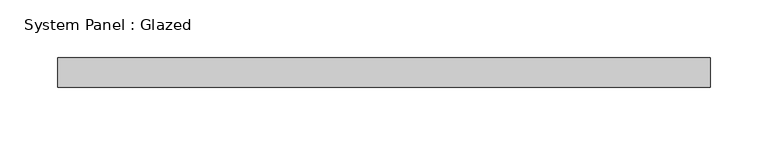
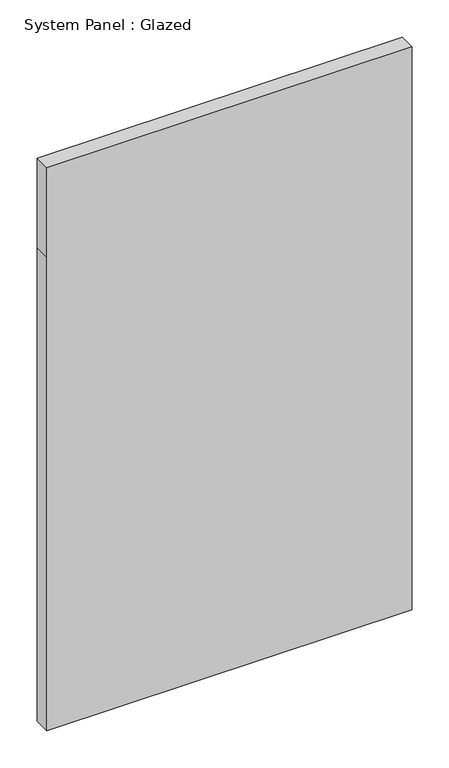
"""IFC4 building model written with IfcOpenShell, lengths in millimetres: plate geometry, System Panel : Glazed."""

from ifc_helpers import new_model, si_unit, frame, origin, place, context, project, spatial, polyline, outline, extrude, source, transform, mapped, element, save


def system_panel_glazed_a2969b70(model_context):
    return source(origin(), model_context, "Body", "SweptSolid", [
        extrude(outline(polyline([(0.0, -282.575), (0.0, 282.575), (774.7, 282.575), (920.75, 282.575), (920.75, -282.575), (774.7, -282.575), (0.0, -282.575)])), frame((0.0, 19.05, 0.0), z_axis=(0.0, 1.0, 0.0), x_axis=(0.0, 0.0, 1.0)), (0.0, 0.0, 1.0), 25.4),
    ])


if __name__ == "__main__":
    model = new_model("IFC4")
    model_context = context("Model", 3, world=origin())
    ifc_project = project(units=[si_unit("LENGTHUNIT", "METRE", prefix="MILLI")], contexts=[model_context])
    site = spatial("IfcSite", under=ifc_project)
    building = spatial("IfcBuilding", under=site)
    placement = place(None, origin())
    system_panel_glazed_shape = system_panel_glazed_a2969b70(model_context)
    element("IfcPlate", 1, ObjectType="System Panel : Glazed", at=placement, inside=building, context=model_context, shape_type="MappedRepresentation", body=[
        mapped(system_panel_glazed_shape, transform((0.0, 0.0, 0.0), x_axis=(1.0, 0.0, 0.0), y_axis=(0.0, 1.0, 0.0), z_axis=(0.0, 0.0, 1.0))),
    ])
    save(model, "model.ifc")

# Revit data of these elements
# Type "System Panel : Glazed"
#   Construction Type Id = "GSP4R"
#   Analytic Construction = "1/8 in Pilkington single glazing"
#   Visual Light Transmittance = 0.9
#   Solar Heat Gain Coefficient = 0.86
#   Heat Transfer Coefficient (U) = 1.18115 BTU/(h·ft²·°F)
#   Define Thermal Properties by = 1
# Element 1 (IfcPlate, "System Panel : Glazed")
#   Materials on its faces: "Glass"
# Materials
#   "Glass": class "Glass", colour RGB 0 128 192, transparency 0.75, Description = "Soda Lime Glass", Cost = 0
